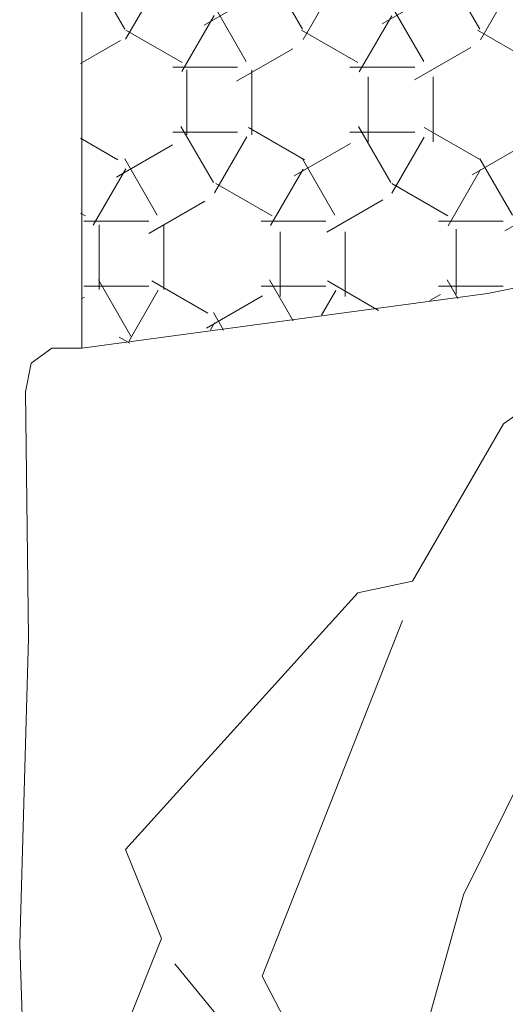
# Model space of a CAD drawing. Units: inches. Extents: x 1994 to 3075, y 3517 to 3950.
# Tile 36 of 58: x 1994.62919 to 1994.63804, y 3553.7375 to 3553.75542. Entities that reach past the tile are written whole.
import ezdxf

# ---------------------------------------------------------------- set-up
doc = ezdxf.new("R2010")
doc.units = ezdxf.units.IN
doc.layers.add('A-FURN-REFR', color=8, linetype='Continuous', lineweight=13)
doc.layers.add('A-FURN-REFR-PATT', color=8, linetype='Continuous', lineweight=13)

msp = doc.modelspace()

# ---------------------------------------------------------------- hatches: boundary and pattern name
at = {"layer": 'A-FURN-REFR-PATT'}
h = msp.add_hatch(dxfattribs=at)
h.set_pattern_fill('ESA_QT1', color=256, scale=0.001181, style=0, pattern_type=2)
h.set_pattern_definition([(0, (2000.7131367, 3549.95567), (0.0016133858, 0.0027944882), [0.0011811024, -0.0020457874]), (0, (2000.7131367, 3549.956851), (0.0016133858, 0.0027944882), [0.0011811024, -0.0020457874]), (60, (2000.7147507, 3549.9540566), (-0.0016134048, 0.0027944772), [0.0011811024, -0.0020457874]), (60, (2000.7137272, 3549.9546472), (-0.0016134048, 0.0027944772), [0.0011811024, -0.0020457874]), (120, (2000.7159311, 3549.9540566), (-0.0032267907, -1.1e-08), [0.0011811024, -0.0020457874]), (120, (2000.716954, 3549.9546472), (-0.0032267907, -1.1e-08), [0.0011811024, -0.0020457874]), (90, (2000.7131367, 3549.95567), (-0.00161338583, 0.0027944882), [0.0011811024, -0.0044079921]), (90, (2000.7143178, 3549.95567), (-0.00161338583, 0.0027944882), [0.0011811024, -0.0044079921]), (30, (2000.7159311, 3549.9540566), (0.00161340485, 0.0027944772), [0.0011811024, -0.0044079921]), (150, (2000.71475, 3549.9540566), (-0.00322679068, 1.1e-08), [0.0011811024, -0.0044079921]), (30, (2000.7153406, 3549.9550795), (0.00161340485, 0.0027944772), [0.0011811024, -0.0044079921]), (150, (2000.7153406, 3549.9550795), (-0.00322679068, 1.1e-08), [0.0011811024, -0.0044079921])])
edge = h.paths.add_edge_path()
edge.add_ellipse((1994.640876, 3553.752584), major_axis=(0, 0.019971), ratio=0.910403, start_angle=279.2385, end_angle=295.7126)
edge.add_ellipse((1994.661382, 3553.784799), major_axis=(0, 0.024564), ratio=0.910403, start_angle=170.9484, end_angle=180.8636)
edge.add_line((1994.661753, 3553.760238), (1994.660448, 3553.761168))
edge.add_line((1994.660448, 3553.761168), (1994.657839, 3553.762473))
edge.add_line((1994.657839, 3553.762473), (1994.656621, 3553.763504))
edge.add_line((1994.656621, 3553.763504), (1994.655861, 3553.763272))
edge.add_line((1994.655861, 3553.763272), (1994.655293, 3553.763476))
edge.add_line((1994.655293, 3553.763476), (1994.655493, 3553.762522))
edge.add_line((1994.655493, 3553.762522), (1994.655292, 3553.760584))
edge.add_line((1994.655292, 3553.760584), (1994.655292, 3553.760424))
edge.add_line((1994.655292, 3553.760424), (1994.655994, 3553.759788))
edge.add_line((1994.655994, 3553.759788), (1994.656079, 3553.758256))
edge.add_line((1994.656079, 3553.758256), (1994.654831, 3553.75802))
edge.add_line((1994.654831, 3553.75802), (1994.653607, 3553.75863))
edge.add_line((1994.653607, 3553.75863), (1994.651194, 3553.757931))
edge.add_line((1994.651194, 3553.757931), (1994.647697, 3553.757851))
edge.add_line((1994.647697, 3553.757851), (1994.645839, 3553.758008))
edge.add_line((1994.645839, 3553.758008), (1994.644836, 3553.757661))
edge.add_line((1994.644836, 3553.757661), (1994.64177, 3553.757379))
edge.add_line((1994.64177, 3553.757379), (1994.63952, 3553.757537))
edge.add_line((1994.63952, 3553.757537), (1994.636664, 3553.757269))
edge.add_line((1994.636664, 3553.757269), (1994.635142, 3553.757511))
edge.add_line((1994.635142, 3553.757511), (1994.634583, 3553.7569))
edge.add_line((1994.634583, 3553.7569), (1994.633061, 3553.756568))
edge.add_line((1994.633061, 3553.756568), (1994.631936, 3553.756647))
edge.add_line((1994.631936, 3553.756647), (1994.631946, 3553.757723))
edge.add_line((1994.631946, 3553.757723), (1994.632293, 3553.759053))
edge.add_line((1994.632293, 3553.759053), (1994.631942, 3553.760336))
edge.add_line((1994.631942, 3553.760336), (1994.631857, 3553.761868))
edge.add_line((1994.631857, 3553.761868), (1994.63213, 3553.76327))
edge.add_line((1994.63213, 3553.76327), (1994.632168, 3553.765117))
edge.add_line((1994.632168, 3553.765117), (1994.631874, 3553.766635))
edge.add_line((1994.631874, 3553.766635), (1994.632212, 3553.768118))
edge.add_line((1994.632212, 3553.768118), (1994.631521, 3553.769225))
edge.add_line((1994.631521, 3553.769225), (1994.631256, 3553.770206))
edge.add_line((1994.631256, 3553.770206), (1994.631719, 3553.770698))
edge.add_line((1994.631719, 3553.770698), (1994.632688, 3553.770917))
edge.add_line((1994.632688, 3553.770917), (1994.633747, 3553.770757))
edge.add_line((1994.633747, 3553.770757), (1994.63499, 3553.77107))
edge.add_line((1994.63499, 3553.77107), (1994.637864, 3553.771031))
edge.add_line((1994.637864, 3553.771031), (1994.638857, 3553.770678))
edge.add_line((1994.638857, 3553.770678), (1994.641165, 3553.770867))
edge.add_line((1994.641165, 3553.770867), (1994.645224, 3553.770907))
edge.add_line((1994.645224, 3553.770907), (1994.645865, 3553.770719))
edge.add_line((1994.645865, 3553.770719), (1994.647785, 3553.771462))
edge.add_line((1994.647785, 3553.771462), (1994.650215, 3553.771855))
edge.add_line((1994.650215, 3553.771855), (1994.65289, 3553.771785))
edge.add_line((1994.65289, 3553.771785), (1994.653416, 3553.772222))
edge.add_line((1994.653416, 3553.772222), (1994.654716, 3553.77277))
edge.add_line((1994.654716, 3553.77277), (1994.655776, 3553.77261))
edge.add_line((1994.655776, 3553.77261), (1994.655708, 3553.771299))
edge.add_line((1994.655708, 3553.771299), (1994.655135, 3553.770261))
edge.add_line((1994.655135, 3553.770261), (1994.655243, 3553.769577))
edge.add_line((1994.655243, 3553.769577), (1994.655057, 3553.767873))
edge.add_line((1994.655057, 3553.767873), (1994.655113, 3553.767736))
edge.add_line((1994.655113, 3553.767736), (1994.655702, 3553.76907))
edge.add_line((1994.655702, 3553.76907), (1994.656565, 3553.770145))
edge.add_line((1994.656565, 3553.770145), (1994.657423, 3553.771734))
edge.add_line((1994.657423, 3553.771734), (1994.657844, 3553.773215))
edge.add_line((1994.657844, 3553.773215), (1994.658028, 3553.77343))
edge.add_line((1994.658028, 3553.77343), (1994.632244, 3553.77343))
edge.add_ellipse((1994.632244, 3553.771319), major_axis=(0, 0.002111), ratio=0.910403, start_angle=0, end_angle=90)
edge.add_line((1994.630322, 3553.771319), (1994.630322, 3553.749441))
edge.add_line((1994.630322, 3553.749441), (1994.637709, 3553.750433))
edge.add_line((1994.637709, 3553.750433), (1994.645849, 3553.752088))
edge.add_line((1994.645849, 3553.752088), (1994.649254, 3553.75227))
edge.add_line((1994.649254, 3553.75227), (1994.654398, 3553.752423))
edge.add_line((1994.654398, 3553.752423), (1994.656593, 3553.752621))
edge.add_ellipse((1994.639937, 3553.760628), major_axis=(0, 0.019971), ratio=0.910403, start_angle=244.323, end_angle=253.1594)
edge.add_ellipse((1994.674344, 3553.771437), major_axis=(0, 0.024564), ratio=0.910403, start_angle=133.6721, end_angle=139.6806)
edge.add_line((1994.659095, 3553.753469), (1994.658861, 3553.755509))
edge = h.paths.add_edge_path()
edge.add_ellipse((1994.680284, 3553.771319), major_axis=(0, 0.002111), ratio=0.910403, start_angle=270, end_angle=360)
edge.add_line((1994.680284, 3553.77343), (1994.665356, 3553.77343))
edge.add_line((1994.665356, 3553.77343), (1994.665734, 3553.77298))
edge.add_line((1994.665734, 3553.77298), (1994.66783, 3553.771902))
edge.add_line((1994.66783, 3553.771902), (1994.671387, 3553.769751))
edge.add_line((1994.671387, 3553.769751), (1994.671861, 3553.769242))
edge.add_line((1994.671861, 3553.769242), (1994.673866, 3553.768856))
edge.add_line((1994.673866, 3553.768856), (1994.676159, 3553.76789))
edge.add_line((1994.676159, 3553.76789), (1994.67846, 3553.766389))
edge.add_line((1994.67846, 3553.766389), (1994.679113, 3553.766487))
edge.add_line((1994.679113, 3553.766487), (1994.680491, 3553.766264))
edge.add_line((1994.680491, 3553.766264), (1994.681343, 3553.765554))
edge.add_line((1994.681343, 3553.765554), (1994.680699, 3553.764448))
edge.add_line((1994.680699, 3553.764448), (1994.679737, 3553.763852))
edge.add_line((1994.679737, 3553.763852), (1994.679525, 3553.763197))
edge.add_line((1994.679525, 3553.763197), (1994.678603, 3553.761813))
edge.add_line((1994.678603, 3553.761813), (1994.678548, 3553.76116))
edge.add_line((1994.678548, 3553.76116), (1994.678066, 3553.759541))
edge.add_line((1994.678066, 3553.759541), (1994.676936, 3553.75803))
edge.add_line((1994.676936, 3553.75803), (1994.676848, 3553.757857))
edge.add_line((1994.676848, 3553.757857), (1994.676595, 3553.756914))
edge.add_line((1994.676595, 3553.756914), (1994.675477, 3553.755213))
edge.add_line((1994.675477, 3553.755213), (1994.675812, 3553.754261))
edge.add_line((1994.675812, 3553.754261), (1994.675202, 3553.75288))
edge.add_line((1994.675202, 3553.75288), (1994.674009, 3553.753346))
edge.add_line((1994.674009, 3553.753346), (1994.673214, 3553.754537))
edge.add_line((1994.673214, 3553.754537), (1994.670799, 3553.755226))
edge.add_line((1994.670799, 3553.755226), (1994.66897, 3553.756302))
edge.add_ellipse((1994.691382, 3553.757287), major_axis=(0, 0.024638), ratio=0.910403, start_angle=92.5166, end_angle=102.9728)
edge.add_line((1994.66943, 3553.75223), (1994.673814, 3553.75171))
edge.add_line((1994.673814, 3553.75171), (1994.677653, 3553.751587))
edge.add_line((1994.677653, 3553.751587), (1994.682205, 3553.751587))
edge.add_line((1994.682205, 3553.751587), (1994.682205, 3553.755102))
edge.add_line((1994.682205, 3553.755102), (1994.682205, 3553.771319))

# ---------------------------------------------------------------- linework, layer by layer
at = {"layer": 'A-FURN-REFR'}
for p, q in [((1994.630322, 3553.749441), (1994.630322, 3553.771319)), ((1994.637709, 3553.750433), (1994.645849, 3553.752088)), ((1994.630322, 3553.749441), (1994.637709, 3553.750433)), ((1994.638001, 3553.748064), (1994.640431, 3553.749786)), ((1994.629778, 3553.749441), (1994.629403, 3553.749166)), ((1994.629778, 3553.749441), (1994.630323, 3553.749441)), ((1994.629403, 3553.749166), (1994.629298, 3553.748648)), ((1994.629298, 3553.748648), (1994.629351, 3553.744162)), ((1994.636345, 3553.745202), (1994.638001, 3553.748064)), ((1994.635349, 3553.744986), (1994.636345, 3553.745202)), ((1994.631123, 3553.740315), (1994.635349, 3553.744986)), ((1994.633608, 3553.738012), (1994.636165, 3553.744481)), ((1994.629351, 3553.744162), (1994.629193, 3553.738583)), ((1994.639169, 3553.743315), (1994.637273, 3553.739491)), ((1994.631778, 3553.738695), (1994.631123, 3553.740315)), ((1994.637273, 3553.739491), (1994.636173, 3553.735557)), ((1994.629921, 3553.734084), (1994.631778, 3553.738695)), ((1994.629193, 3553.738583), (1994.629381, 3553.732902)), ((1994.632016, 3553.738235), (1994.634003, 3553.735824)), ((1994.634482, 3553.736326), (1994.633608, 3553.738012))]:
    msp.add_line(p, q, dxfattribs=at)

doc.saveas('drawing.dxf')
